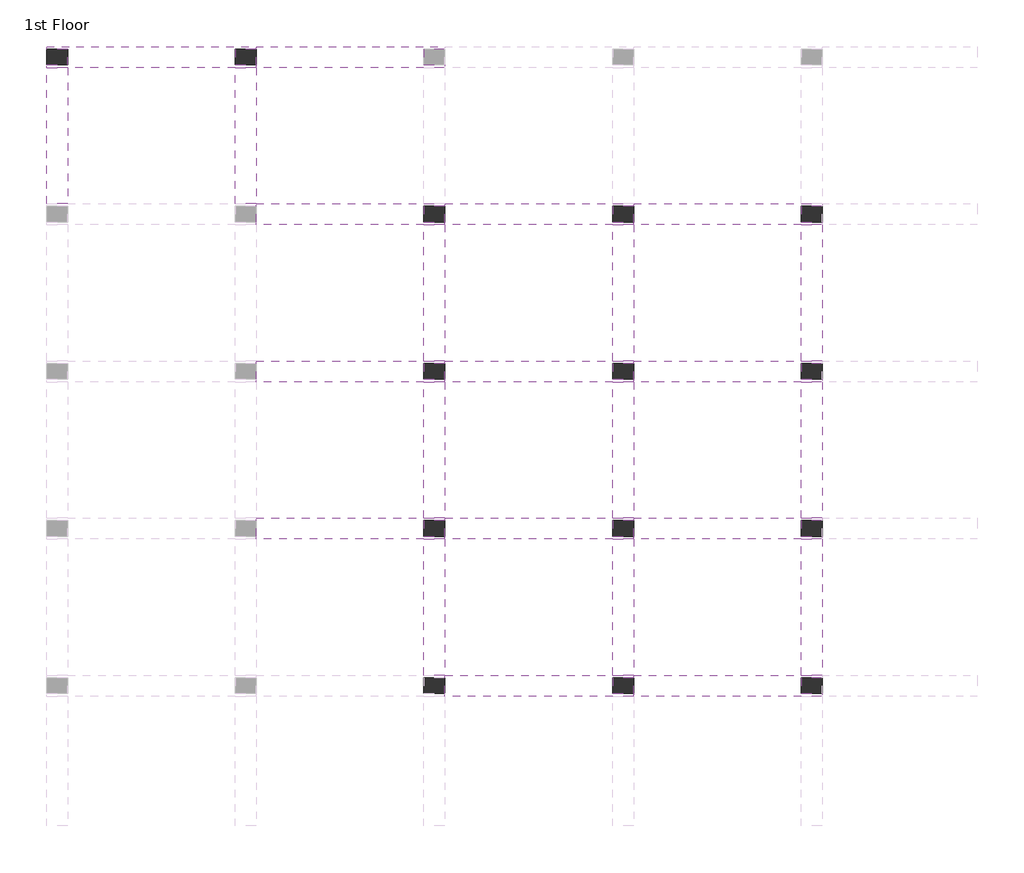
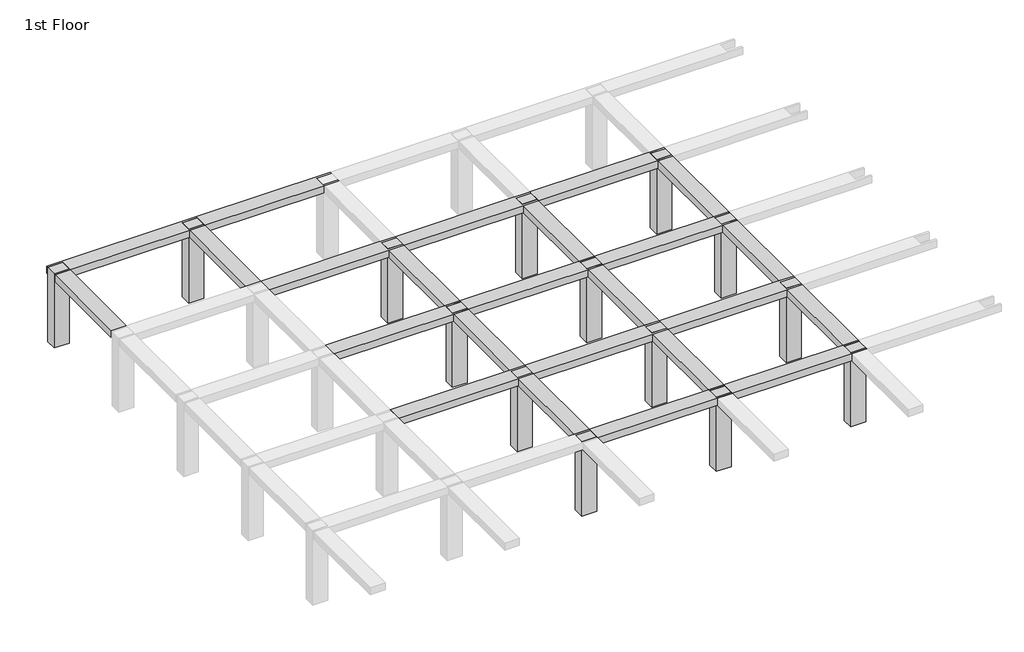
# One storey, part 2 of 3: 24 beams, 14 columns.
"""IFC4 building model written with IfcOpenShell, lengths in millimetres."""

from ifc_helpers import new_model, si_unit, frame, origin, place, context, project, spatial, polyline, outline, extrude, faceted_brep, element, save

model = new_model("IFC4")

# Units and contexts
model_context = context("Model", 3, world=origin())
ifc_project = project(units=[si_unit("LENGTHUNIT", "METRE", prefix="MILLI")], contexts=[model_context])

# Site, building, storey
site = spatial("IfcSite", under=ifc_project)
building = spatial("IfcBuilding", under=site)
storey = spatial("IfcBuildingStorey", under=building, Name="1st Floor", Elevation=3200.4)

# Beams
placement = place(None, origin())
element("IfcBeam", 1, ObjectType="Concrete-Rectangular Beam : 2' x2'", at=placement, inside=storey, context=model_context, shape_type="Brep", body=[
    faceted_brep([(-5646.474232, 1680.7831222, 6400.8), (-6256.074232, 1680.7831222, 6400.8), (-11132.874232, 1680.7831222, 6400.8), (-11132.874232, 1604.5831222, 6400.8), (-11132.874232, 1147.3831222, 6400.8), (-11132.874232, 1071.1831222, 6400.8), (-6256.074232, 1071.1831222, 6400.8), (-5646.474232, 1071.1831222, 6400.8), (-5646.474232, 1147.3831222, 6400.8), (-6256.074232, 1147.3831222, 6400.8), (-6256.074232, 1604.5831222, 6400.8), (-5646.474232, 1604.5831222, 6400.8), (-5646.474232, 1071.1831222, 6096.0), (-11132.874232, 1071.1831222, 6096.0), (-6256.074232, 1071.1831222, 6096.0), (-11132.874232, 1147.3831222, 6096.0), (-11132.874232, 1604.5831222, 6096.0), (-11132.874232, 1680.7831222, 6096.0), (-6256.074232, 1680.7831222, 6096.0), (-5646.474232, 1680.7831222, 6096.0), (-5646.474232, 1604.5831222, 6096.0), (-6256.074232, 1604.5831222, 6096.0), (-6256.074232, 1147.3831222, 6096.0), (-5646.474232, 1147.3831222, 6096.0)], [[[0, 1, 2, 3, 4, 5, 6, 7, 8, 9, 10, 11]], [[12, 7, 6, 5, 13, 14]], [[12, 14, 13, 15, 16, 17, 18, 19, 20, 21, 22, 23]], [[0, 19, 18, 17, 2, 1]], [[7, 12, 23, 8]], [[5, 4, 3, 2, 17, 16, 15, 13]], [[22, 9, 8, 23]], [[9, 22, 21, 10]], [[10, 21, 20, 11]], [[19, 0, 11, 20]]]),
])
element("IfcBeam", 2, ObjectType="Concrete-Rectangular Beam : 2' x2'", at=placement, inside=storey, context=model_context, shape_type="Brep", body=[
    faceted_brep([(-5646.474232, 1680.7831222, 6400.8), (-5646.474232, 1604.5831222, 6400.8), (-5646.474232, 1147.3831222, 6400.8), (-5646.474232, 1071.1831222, 6400.8), (-769.674232, 1071.1831222, 6400.8), (-160.074232, 1071.1831222, 6400.8), (-160.074232, 1147.3831222, 6400.8), (-769.674232, 1147.3831222, 6400.8), (-769.674232, 1604.5831222, 6400.8), (-160.074232, 1604.5831222, 6400.8), (-160.074232, 1680.7831222, 6400.8), (-769.674232, 1680.7831222, 6400.8), (-5646.474232, 1071.1831222, 6096.0), (-769.674232, 1071.1831222, 6096.0), (-160.074232, 1071.1831222, 6096.0), (-5646.474232, 1147.3831222, 6096.0), (-5646.474232, 1604.5831222, 6096.0), (-5646.474232, 1680.7831222, 6096.0), (-769.674232, 1680.7831222, 6096.0), (-160.074232, 1680.7831222, 6096.0), (-160.074232, 1604.5831222, 6096.0), (-769.674232, 1604.5831222, 6096.0), (-769.674232, 1147.3831222, 6096.0), (-160.074232, 1147.3831222, 6096.0)], [[[0, 1, 2, 3, 4, 5, 6, 7, 8, 9, 10, 11]], [[3, 12, 13, 14, 5, 4]], [[12, 15, 16, 17, 18, 19, 20, 21, 22, 23, 14, 13]], [[10, 19, 18, 17, 0, 11]], [[3, 2, 1, 0, 17, 16, 15, 12]], [[5, 14, 23, 6]], [[22, 7, 6, 23]], [[7, 22, 21, 8]], [[8, 21, 20, 9]], [[19, 10, 9, 20]]]),
])
element("IfcBeam", 3, ObjectType="Concrete-Rectangular Beam : 2' x2'", at=placement, inside=storey, context=model_context, shape_type="Brep", body=[
    faceted_brep([(-16619.274232, 6252.7831222, 6400.8), (-16619.274232, 6176.5831222, 6400.8), (-16619.274232, 5719.3831222, 6400.8), (-16619.274232, 5643.1831222, 6400.8), (-11742.474232, 5643.1831222, 6400.8), (-11132.874232, 5643.1831222, 6400.8), (-11132.874232, 5719.3831222, 6400.8), (-11742.474232, 5719.3831222, 6400.8), (-11742.474232, 6176.5831222, 6400.8), (-11132.874232, 6176.5831222, 6400.8), (-11132.874232, 6252.7831222, 6400.8), (-11742.474232, 6252.7831222, 6400.8), (-16619.274232, 5643.1831222, 6096.0), (-11742.474232, 5643.1831222, 6096.0), (-11132.874232, 5643.1831222, 6096.0), (-16619.274232, 5719.3831222, 6096.0), (-16619.274232, 6176.5831222, 6096.0), (-16619.274232, 6252.7831222, 6096.0), (-11742.474232, 6252.7831222, 6096.0), (-11132.874232, 6252.7831222, 6096.0), (-11132.874232, 6176.5831222, 6096.0), (-11742.474232, 6176.5831222, 6096.0), (-11742.474232, 5719.3831222, 6096.0), (-11132.874232, 5719.3831222, 6096.0)], [[[0, 1, 2, 3, 4, 5, 6, 7, 8, 9, 10, 11]], [[3, 12, 13, 14, 5, 4]], [[12, 15, 16, 17, 18, 19, 20, 21, 22, 23, 14, 13]], [[10, 19, 18, 17, 0, 11]], [[3, 2, 1, 0, 17, 16, 15, 12]], [[5, 14, 23, 6]], [[22, 7, 6, 23]], [[7, 22, 21, 8]], [[8, 21, 20, 9]], [[19, 10, 9, 20]]]),
])
element("IfcBeam", 4, ObjectType="Concrete-Rectangular Beam : 2' x2'", at=placement, inside=storey, context=model_context, shape_type="Brep", body=[
    faceted_brep([(-5646.474232, 6252.7831222, 6400.8), (-6256.074232, 6252.7831222, 6400.8), (-11132.874232, 6252.7831222, 6400.8), (-11132.874232, 6176.5831222, 6400.8), (-11132.874232, 5719.3831222, 6400.8), (-11132.874232, 5643.1831222, 6400.8), (-6256.074232, 5643.1831222, 6400.8), (-5646.474232, 5643.1831222, 6400.8), (-5646.474232, 5719.3831222, 6400.8), (-6256.074232, 5719.3831222, 6400.8), (-6256.074232, 6176.5831222, 6400.8), (-5646.474232, 6176.5831222, 6400.8), (-5646.474232, 5643.1831222, 6096.0), (-11132.874232, 5643.1831222, 6096.0), (-6256.074232, 5643.1831222, 6096.0), (-11132.874232, 5719.3831222, 6096.0), (-11132.874232, 6176.5831222, 6096.0), (-11132.874232, 6252.7831222, 6096.0), (-6256.074232, 6252.7831222, 6096.0), (-5646.474232, 6252.7831222, 6096.0), (-5646.474232, 6176.5831222, 6096.0), (-6256.074232, 6176.5831222, 6096.0), (-6256.074232, 5719.3831222, 6096.0), (-5646.474232, 5719.3831222, 6096.0)], [[[0, 1, 2, 3, 4, 5, 6, 7, 8, 9, 10, 11]], [[12, 7, 6, 5, 13, 14]], [[12, 14, 13, 15, 16, 17, 18, 19, 20, 21, 22, 23]], [[0, 19, 18, 17, 2, 1]], [[7, 12, 23, 8]], [[5, 4, 3, 2, 17, 16, 15, 13]], [[22, 9, 8, 23]], [[9, 22, 21, 10]], [[10, 21, 20, 11]], [[19, 0, 11, 20]]]),
])
element("IfcBeam", 5, ObjectType="Concrete-Rectangular Beam : 2' x2'", at=placement, inside=storey, context=model_context, shape_type="Brep", body=[
    faceted_brep([(-5646.474232, 6252.7831222, 6400.8), (-5646.474232, 6176.5831222, 6400.8), (-5646.474232, 5719.3831222, 6400.8), (-5646.474232, 5643.1831222, 6400.8), (-769.674232, 5643.1831222, 6400.8), (-160.074232, 5643.1831222, 6400.8), (-160.074232, 5719.3831222, 6400.8), (-769.674232, 5719.3831222, 6400.8), (-769.674232, 6176.5831222, 6400.8), (-160.074232, 6176.5831222, 6400.8), (-160.074232, 6252.7831222, 6400.8), (-769.674232, 6252.7831222, 6400.8), (-5646.474232, 5643.1831222, 6096.0), (-769.674232, 5643.1831222, 6096.0), (-160.074232, 5643.1831222, 6096.0), (-5646.474232, 5719.3831222, 6096.0), (-5646.474232, 6176.5831222, 6096.0), (-5646.474232, 6252.7831222, 6096.0), (-769.674232, 6252.7831222, 6096.0), (-160.074232, 6252.7831222, 6096.0), (-160.074232, 6176.5831222, 6096.0), (-769.674232, 6176.5831222, 6096.0), (-769.674232, 5719.3831222, 6096.0), (-160.074232, 5719.3831222, 6096.0)], [[[0, 1, 2, 3, 4, 5, 6, 7, 8, 9, 10, 11]], [[3, 12, 13, 14, 5, 4]], [[12, 15, 16, 17, 18, 19, 20, 21, 22, 23, 14, 13]], [[10, 19, 18, 17, 0, 11]], [[3, 2, 1, 0, 17, 16, 15, 12]], [[5, 14, 23, 6]], [[22, 7, 6, 23]], [[7, 22, 21, 8]], [[8, 21, 20, 9]], [[19, 10, 9, 20]]]),
])
element("IfcBeam", 6, ObjectType="Concrete-Rectangular Beam : 2' x2'", at=placement, inside=storey, context=model_context, shape_type="Brep", body=[
    faceted_brep([(-16619.274232, 10824.7831222, 6400.8), (-16619.274232, 10748.5831222, 6400.8), (-16619.274232, 10291.3831222, 6400.8), (-16619.274232, 10215.1831222, 6400.8), (-11742.474232, 10215.1831222, 6400.8), (-11132.874232, 10215.1831222, 6400.8), (-11132.874232, 10291.3831222, 6400.8), (-11742.474232, 10291.3831222, 6400.8), (-11742.474232, 10748.5831222, 6400.8), (-11132.874232, 10748.5831222, 6400.8), (-11132.874232, 10824.7831222, 6400.8), (-11742.474232, 10824.7831222, 6400.8), (-16619.274232, 10215.1831222, 6096.0), (-11742.474232, 10215.1831222, 6096.0), (-11132.874232, 10215.1831222, 6096.0), (-16619.274232, 10291.3831222, 6096.0), (-16619.274232, 10748.5831222, 6096.0), (-16619.274232, 10824.7831222, 6096.0), (-11742.474232, 10824.7831222, 6096.0), (-11132.874232, 10824.7831222, 6096.0), (-11132.874232, 10748.5831222, 6096.0), (-11742.474232, 10748.5831222, 6096.0), (-11742.474232, 10291.3831222, 6096.0), (-11132.874232, 10291.3831222, 6096.0)], [[[0, 1, 2, 3, 4, 5, 6, 7, 8, 9, 10, 11]], [[3, 12, 13, 14, 5, 4]], [[12, 15, 16, 17, 18, 19, 20, 21, 22, 23, 14, 13]], [[10, 19, 18, 17, 0, 11]], [[3, 2, 1, 0, 17, 16, 15, 12]], [[5, 14, 23, 6]], [[22, 7, 6, 23]], [[7, 22, 21, 8]], [[8, 21, 20, 9]], [[19, 10, 9, 20]]]),
])
element("IfcBeam", 7, ObjectType="Concrete-Rectangular Beam : 2' x2'", at=placement, inside=storey, context=model_context, shape_type="Brep", body=[
    faceted_brep([(-11132.874232, 10824.7831222, 6400.8), (-11132.874232, 10748.5831222, 6400.8), (-11132.874232, 10291.3831222, 6400.8), (-11132.874232, 10215.1831222, 6400.8), (-6256.074232, 10215.1831222, 6400.8), (-5646.474232, 10215.1831222, 6400.8), (-5646.474232, 10291.3831222, 6400.8), (-6256.074232, 10291.3831222, 6400.8), (-6256.074232, 10748.5831222, 6400.8), (-5646.474232, 10748.5831222, 6400.8), (-5646.474232, 10824.7831222, 6400.8), (-6256.074232, 10824.7831222, 6400.8), (-11132.874232, 10215.1831222, 6096.0), (-6256.074232, 10215.1831222, 6096.0), (-5646.474232, 10215.1831222, 6096.0), (-11132.874232, 10291.3831222, 6096.0), (-11132.874232, 10748.5831222, 6096.0), (-11132.874232, 10824.7831222, 6096.0), (-6256.074232, 10824.7831222, 6096.0), (-5646.474232, 10824.7831222, 6096.0), (-5646.474232, 10748.5831222, 6096.0), (-6256.074232, 10748.5831222, 6096.0), (-6256.074232, 10291.3831222, 6096.0), (-5646.474232, 10291.3831222, 6096.0)], [[[0, 1, 2, 3, 4, 5, 6, 7, 8, 9, 10, 11]], [[3, 12, 13, 14, 5, 4]], [[12, 15, 16, 17, 18, 19, 20, 21, 22, 23, 14, 13]], [[10, 19, 18, 17, 0, 11]], [[3, 2, 1, 0, 17, 16, 15, 12]], [[5, 14, 23, 6]], [[22, 7, 6, 23]], [[7, 22, 21, 8]], [[8, 21, 20, 9]], [[19, 10, 9, 20]]]),
])
element("IfcBeam", 8, ObjectType="Concrete-Rectangular Beam : 2' x2'", at=placement, inside=storey, context=model_context, shape_type="Brep", body=[
    faceted_brep([(-5646.474232, 10824.7831222, 6400.8), (-5646.474232, 10748.5831222, 6400.8), (-5646.474232, 10291.3831222, 6400.8), (-5646.474232, 10215.1831222, 6400.8), (-769.674232, 10215.1831222, 6400.8), (-160.074232, 10215.1831222, 6400.8), (-160.074232, 10291.3831222, 6400.8), (-769.674232, 10291.3831222, 6400.8), (-769.674232, 10748.5831222, 6400.8), (-160.074232, 10748.5831222, 6400.8), (-160.074232, 10824.7831222, 6400.8), (-769.674232, 10824.7831222, 6400.8), (-5646.474232, 10215.1831222, 6096.0), (-769.674232, 10215.1831222, 6096.0), (-160.074232, 10215.1831222, 6096.0), (-5646.474232, 10291.3831222, 6096.0), (-5646.474232, 10748.5831222, 6096.0), (-5646.474232, 10824.7831222, 6096.0), (-769.674232, 10824.7831222, 6096.0), (-160.074232, 10824.7831222, 6096.0), (-160.074232, 10748.5831222, 6096.0), (-769.674232, 10748.5831222, 6096.0), (-769.674232, 10291.3831222, 6096.0), (-160.074232, 10291.3831222, 6096.0)], [[[0, 1, 2, 3, 4, 5, 6, 7, 8, 9, 10, 11]], [[3, 12, 13, 14, 5, 4]], [[12, 15, 16, 17, 18, 19, 20, 21, 22, 23, 14, 13]], [[10, 19, 18, 17, 0, 11]], [[3, 2, 1, 0, 17, 16, 15, 12]], [[5, 14, 23, 6]], [[22, 7, 6, 23]], [[7, 22, 21, 8]], [[8, 21, 20, 9]], [[19, 10, 9, 20]]]),
])
element("IfcBeam", 9, ObjectType="Concrete-Rectangular Beam : 2' x2'", at=placement, inside=storey, context=model_context, shape_type="Brep", body=[
    faceted_brep([(-16619.274232, 15396.7831222, 6400.8), (-16619.274232, 15320.5831222, 6400.8), (-16619.274232, 14863.3831222, 6400.8), (-16619.274232, 14787.1831222, 6400.8), (-11742.474232, 14787.1831222, 6400.8), (-11132.874232, 14787.1831222, 6400.8), (-11132.874232, 14863.3831222, 6400.8), (-11742.474232, 14863.3831222, 6400.8), (-11742.474232, 15320.5831222, 6400.8), (-11132.874232, 15320.5831222, 6400.8), (-11132.874232, 15396.7831222, 6400.8), (-11742.474232, 15396.7831222, 6400.8), (-16619.274232, 14787.1831222, 6096.0), (-11742.474232, 14787.1831222, 6096.0), (-11132.874232, 14787.1831222, 6096.0), (-16619.274232, 14863.3831222, 6096.0), (-16619.274232, 15320.5831222, 6096.0), (-16619.274232, 15396.7831222, 6096.0), (-11742.474232, 15396.7831222, 6096.0), (-11132.874232, 15396.7831222, 6096.0), (-11132.874232, 15320.5831222, 6096.0), (-11742.474232, 15320.5831222, 6096.0), (-11742.474232, 14863.3831222, 6096.0), (-11132.874232, 14863.3831222, 6096.0)], [[[0, 1, 2, 3, 4, 5, 6, 7, 8, 9, 10, 11]], [[3, 12, 13, 14, 5, 4]], [[12, 15, 16, 17, 18, 19, 20, 21, 22, 23, 14, 13]], [[10, 19, 18, 17, 0, 11]], [[3, 2, 1, 0, 17, 16, 15, 12]], [[5, 14, 23, 6]], [[22, 7, 6, 23]], [[7, 22, 21, 8]], [[8, 21, 20, 9]], [[19, 10, 9, 20]]]),
])
element("IfcBeam", 10, ObjectType="Concrete-Rectangular Beam : 2' x2'", at=placement, inside=storey, context=model_context, shape_type="Brep", body=[
    faceted_brep([(-11132.874232, 15396.7831222, 6400.8), (-11132.874232, 15320.5831222, 6400.8), (-11132.874232, 14863.3831222, 6400.8), (-11132.874232, 14787.1831222, 6400.8), (-6256.074232, 14787.1831222, 6400.8), (-5646.474232, 14787.1831222, 6400.8), (-5646.474232, 14863.3831222, 6400.8), (-6256.074232, 14863.3831222, 6400.8), (-6256.074232, 15320.5831222, 6400.8), (-5646.474232, 15320.5831222, 6400.8), (-5646.474232, 15396.7831222, 6400.8), (-6256.074232, 15396.7831222, 6400.8), (-11132.874232, 14787.1831222, 6096.0), (-6256.074232, 14787.1831222, 6096.0), (-5646.474232, 14787.1831222, 6096.0), (-11132.874232, 14863.3831222, 6096.0), (-11132.874232, 15320.5831222, 6096.0), (-11132.874232, 15396.7831222, 6096.0), (-6256.074232, 15396.7831222, 6096.0), (-5646.474232, 15396.7831222, 6096.0), (-5646.474232, 15320.5831222, 6096.0), (-6256.074232, 15320.5831222, 6096.0), (-6256.074232, 14863.3831222, 6096.0), (-5646.474232, 14863.3831222, 6096.0)], [[[0, 1, 2, 3, 4, 5, 6, 7, 8, 9, 10, 11]], [[3, 12, 13, 14, 5, 4]], [[12, 15, 16, 17, 18, 19, 20, 21, 22, 23, 14, 13]], [[10, 19, 18, 17, 0, 11]], [[3, 2, 1, 0, 17, 16, 15, 12]], [[5, 14, 23, 6]], [[22, 7, 6, 23]], [[7, 22, 21, 8]], [[8, 21, 20, 9]], [[19, 10, 9, 20]]]),
])
element("IfcBeam", 11, ObjectType="Concrete-Rectangular Beam : 2' x2'", at=placement, inside=storey, context=model_context, shape_type="Brep", body=[
    faceted_brep([(-5646.474232, 15396.7831222, 6400.8), (-5646.474232, 15320.5831222, 6400.8), (-5646.474232, 14863.3831222, 6400.8), (-5646.474232, 14787.1831222, 6400.8), (-769.674232, 14787.1831222, 6400.8), (-160.074232, 14787.1831222, 6400.8), (-160.074232, 14863.3831222, 6400.8), (-769.674232, 14863.3831222, 6400.8), (-769.674232, 15320.5831222, 6400.8), (-160.074232, 15320.5831222, 6400.8), (-160.074232, 15396.7831222, 6400.8), (-769.674232, 15396.7831222, 6400.8), (-5646.474232, 14787.1831222, 6096.0), (-769.674232, 14787.1831222, 6096.0), (-160.074232, 14787.1831222, 6096.0), (-5646.474232, 14863.3831222, 6096.0), (-5646.474232, 15320.5831222, 6096.0), (-5646.474232, 15396.7831222, 6096.0), (-769.674232, 15396.7831222, 6096.0), (-160.074232, 15396.7831222, 6096.0), (-160.074232, 15320.5831222, 6096.0), (-769.674232, 15320.5831222, 6096.0), (-769.674232, 14863.3831222, 6096.0), (-160.074232, 14863.3831222, 6096.0)], [[[0, 1, 2, 3, 4, 5, 6, 7, 8, 9, 10, 11]], [[3, 12, 13, 14, 5, 4]], [[12, 15, 16, 17, 18, 19, 20, 21, 22, 23, 14, 13]], [[10, 19, 18, 17, 0, 11]], [[3, 2, 1, 0, 17, 16, 15, 12]], [[5, 14, 23, 6]], [[22, 7, 6, 23]], [[7, 22, 21, 8]], [[8, 21, 20, 9]], [[19, 10, 9, 20]]]),
])
element("IfcBeam", 12, ObjectType="Concrete-Rectangular Beam : 2' x2'", at=placement, inside=storey, context=model_context, shape_type="Brep", body=[
    faceted_brep([(-16619.274232, 19968.7831222, 6400.8), (-22715.274232, 19968.7831222, 6400.8), (-22715.274232, 19892.5831222, 6400.8), (-22105.674232, 19892.5831222, 6400.8), (-22105.674232, 19435.3831222, 6400.8), (-22715.274232, 19435.3831222, 6400.8), (-22715.274232, 19359.1831222, 6400.8), (-22105.674232, 19359.1831222, 6400.8), (-17228.874232, 19359.1831222, 6400.8), (-16619.274232, 19359.1831222, 6400.8), (-16619.274232, 19435.3831222, 6400.8), (-17228.874232, 19435.3831222, 6400.8), (-17228.874232, 19892.5831222, 6400.8), (-16619.274232, 19892.5831222, 6400.8), (-22715.274232, 19359.1831222, 6096.0), (-22105.674232, 19359.1831222, 6096.0), (-17228.874232, 19359.1831222, 6096.0), (-16619.274232, 19359.1831222, 6096.0), (-22715.274232, 19435.3831222, 6096.0), (-22105.674232, 19435.3831222, 6096.0), (-22105.674232, 19892.5831222, 6096.0), (-22715.274232, 19892.5831222, 6096.0), (-22715.274232, 19968.7831222, 6096.0), (-16619.274232, 19968.7831222, 6096.0), (-16619.274232, 19892.5831222, 6096.0), (-17228.874232, 19892.5831222, 6096.0), (-17228.874232, 19435.3831222, 6096.0), (-16619.274232, 19435.3831222, 6096.0)], [[[0, 1, 2, 3, 4, 5, 6, 7, 8, 9, 10, 11, 12, 13]], [[6, 14, 15, 16, 17, 9, 8, 7]], [[17, 16, 15, 14, 18, 19, 20, 21, 22, 23, 24, 25, 26, 27]], [[22, 1, 0, 23]], [[14, 6, 5, 18]], [[9, 17, 27, 10]], [[19, 4, 3, 20]], [[4, 19, 18, 5]], [[20, 3, 2, 21]], [[1, 22, 21, 2]], [[26, 11, 10, 27]], [[11, 26, 25, 12]], [[12, 25, 24, 13]], [[23, 0, 13, 24]]]),
])
element("IfcBeam", 13, ObjectType="Concrete-Rectangular Beam : 2' x2'", at=placement, inside=storey, context=model_context, shape_type="Brep", body=[
    faceted_brep([(-11132.874232, 19968.7831222, 6400.8), (-16619.274232, 19968.7831222, 6400.8), (-16619.274232, 19892.5831222, 6400.8), (-16619.274232, 19435.3831222, 6400.8), (-16619.274232, 19359.1831222, 6400.8), (-11742.474232, 19359.1831222, 6400.8), (-11132.874232, 19359.1831222, 6400.8), (-11132.874232, 19435.3831222, 6400.8), (-11742.474232, 19435.3831222, 6400.8), (-11742.474232, 19892.5831222, 6400.8), (-11132.874232, 19892.5831222, 6400.8), (-11132.874232, 19359.1831222, 6096.0), (-16619.274232, 19359.1831222, 6096.0), (-11742.474232, 19359.1831222, 6096.0), (-16619.274232, 19435.3831222, 6096.0), (-16619.274232, 19892.5831222, 6096.0), (-16619.274232, 19968.7831222, 6096.0), (-11132.874232, 19968.7831222, 6096.0), (-11132.874232, 19892.5831222, 6096.0), (-11742.474232, 19892.5831222, 6096.0), (-11742.474232, 19435.3831222, 6096.0), (-11132.874232, 19435.3831222, 6096.0)], [[[0, 1, 2, 3, 4, 5, 6, 7, 8, 9, 10]], [[11, 6, 5, 4, 12, 13]], [[11, 13, 12, 14, 15, 16, 17, 18, 19, 20, 21]], [[0, 17, 16, 1]], [[6, 11, 21, 7]], [[4, 3, 2, 1, 16, 15, 14, 12]], [[20, 8, 7, 21]], [[8, 20, 19, 9]], [[9, 19, 18, 10]], [[17, 0, 10, 18]]]),
])
element("IfcBeam", 14, ObjectType="Concrete-Rectangular Beam : 2' x2'", at=placement, inside=storey, context=model_context, shape_type="SweptSolid", body=[
    extrude(outline(polyline([(-22105.674232, 15396.7831222), (-22715.274232, 15396.7831222), (-22715.274232, 19359.1831222), (-22105.674232, 19359.1831222), (-22105.674232, 15396.7831222)])), frame((0.0, 0.0, 6096.0), z_axis=(0.0, 0.0, 1.0), x_axis=(1.0, 0.0, 0.0)), (0.0, 0.0, 1.0), 304.8),
])
element("IfcBeam", 15, ObjectType="Concrete-Rectangular Beam : 2' x2'", at=placement, inside=storey, context=model_context, shape_type="SweptSolid", body=[
    extrude(outline(polyline([(-16619.274232, 15396.7831222), (-17228.874232, 15396.7831222), (-17228.874232, 19359.1831222), (-16619.274232, 19359.1831222), (-16619.274232, 15396.7831222)])), frame((0.0, 0.0, 6096.0), z_axis=(0.0, 0.0, 1.0), x_axis=(1.0, 0.0, 0.0)), (0.0, 0.0, 1.0), 304.8),
])
element("IfcBeam", 16, ObjectType="Concrete-Rectangular Beam : 2' x2'", at=placement, inside=storey, context=model_context, shape_type="SweptSolid", body=[
    extrude(outline(polyline([(-11132.874232, 1680.7831222), (-11742.474232, 1680.7831222), (-11742.474232, 5643.1831222), (-11132.874232, 5643.1831222), (-11132.874232, 1680.7831222)])), frame((0.0, 0.0, 6096.0), z_axis=(0.0, 0.0, 1.0), x_axis=(1.0, 0.0, 0.0)), (0.0, 0.0, 1.0), 304.8),
])
element("IfcBeam", 17, ObjectType="Concrete-Rectangular Beam : 2' x2'", at=placement, inside=storey, context=model_context, shape_type="SweptSolid", body=[
    extrude(outline(polyline([(-11132.874232, 6252.7831222), (-11742.474232, 6252.7831222), (-11742.474232, 10215.1831222), (-11132.874232, 10215.1831222), (-11132.874232, 6252.7831222)])), frame((0.0, 0.0, 6096.0), z_axis=(0.0, 0.0, 1.0), x_axis=(1.0, 0.0, 0.0)), (0.0, 0.0, 1.0), 304.8),
])
element("IfcBeam", 18, ObjectType="Concrete-Rectangular Beam : 2' x2'", at=placement, inside=storey, context=model_context, shape_type="SweptSolid", body=[
    extrude(outline(polyline([(-11132.874232, 10824.7831222), (-11742.474232, 10824.7831222), (-11742.474232, 14787.1831222), (-11132.874232, 14787.1831222), (-11132.874232, 10824.7831222)])), frame((0.0, 0.0, 6096.0), z_axis=(0.0, 0.0, 1.0), x_axis=(1.0, 0.0, 0.0)), (0.0, 0.0, 1.0), 304.8),
])
element("IfcBeam", 19, ObjectType="Concrete-Rectangular Beam : 2' x2'", at=placement, inside=storey, context=model_context, shape_type="SweptSolid", body=[
    extrude(outline(polyline([(-5646.474232, 1680.7831222), (-6256.074232, 1680.7831222), (-6256.074232, 5643.1831222), (-5646.474232, 5643.1831222), (-5646.474232, 1680.7831222)])), frame((0.0, 0.0, 6096.0), z_axis=(0.0, 0.0, 1.0), x_axis=(1.0, 0.0, 0.0)), (0.0, 0.0, 1.0), 304.8),
])
element("IfcBeam", 20, ObjectType="Concrete-Rectangular Beam : 2' x2'", at=placement, inside=storey, context=model_context, shape_type="SweptSolid", body=[
    extrude(outline(polyline([(-5646.474232, 6252.7831222), (-6256.074232, 6252.7831222), (-6256.074232, 10215.1831222), (-5646.474232, 10215.1831222), (-5646.474232, 6252.7831222)])), frame((0.0, 0.0, 6096.0), z_axis=(0.0, 0.0, 1.0), x_axis=(1.0, 0.0, 0.0)), (0.0, 0.0, 1.0), 304.8),
])
element("IfcBeam", 21, ObjectType="Concrete-Rectangular Beam : 2' x2'", at=placement, inside=storey, context=model_context, shape_type="SweptSolid", body=[
    extrude(outline(polyline([(-5646.474232, 10824.7831222), (-6256.074232, 10824.7831222), (-6256.074232, 14787.1831222), (-5646.474232, 14787.1831222), (-5646.474232, 10824.7831222)])), frame((0.0, 0.0, 6096.0), z_axis=(0.0, 0.0, 1.0), x_axis=(1.0, 0.0, 0.0)), (0.0, 0.0, 1.0), 304.8),
])
element("IfcBeam", 22, ObjectType="Concrete-Rectangular Beam : 2' x2'", at=placement, inside=storey, context=model_context, shape_type="SweptSolid", body=[
    extrude(outline(polyline([(-769.674232, 5643.1831222), (-160.074232, 5643.1831222), (-160.074232, 1680.7831222), (-769.674232, 1680.7831222), (-769.674232, 5643.1831222)])), frame((0.0, 0.0, 6096.0), z_axis=(0.0, 0.0, 1.0), x_axis=(1.0, 0.0, 0.0)), (0.0, 0.0, 1.0), 304.8),
])
element("IfcBeam", 23, ObjectType="Concrete-Rectangular Beam : 2' x2'", at=placement, inside=storey, context=model_context, shape_type="SweptSolid", body=[
    extrude(outline(polyline([(-160.074232, 6252.7831222), (-769.674232, 6252.7831222), (-769.674232, 10215.1831222), (-160.074232, 10215.1831222), (-160.074232, 6252.7831222)])), frame((0.0, 0.0, 6096.0), z_axis=(0.0, 0.0, 1.0), x_axis=(1.0, 0.0, 0.0)), (0.0, 0.0, 1.0), 304.8),
])
element("IfcBeam", 24, ObjectType="Concrete-Rectangular Beam : 2' x2'", at=placement, inside=storey, context=model_context, shape_type="SweptSolid", body=[
    extrude(outline(polyline([(-769.674232, 14787.1831222), (-160.074232, 14787.1831222), (-160.074232, 10824.7831222), (-769.674232, 10824.7831222), (-769.674232, 14787.1831222)])), frame((0.0, 0.0, 6096.0), z_axis=(0.0, 0.0, 1.0), x_axis=(1.0, 0.0, 0.0)), (0.0, 0.0, 1.0), 304.8),
])

# Columns
element("IfcColumn", 25, ObjectType="Concrete-Rectangular-Column : 12 x 18", at=placement, inside=storey, context=model_context, shape_type="SweptSolid", body=[
    extrude(outline(polyline([(-11132.874232, 1604.5831222), (-11132.874232, 1147.3831222), (-11742.474232, 1147.3831222), (-11742.474232, 1604.5831222), (-11132.874232, 1604.5831222)])), frame((0.0, 0.0, 3200.4), z_axis=(0.0, 0.0, 1.0), x_axis=(1.0, 0.0, 0.0)), (0.0, 0.0, 1.0), 3200.4),
])
element("IfcColumn", 26, ObjectType="Concrete-Rectangular-Column : 12 x 18", at=placement, inside=storey, context=model_context, shape_type="SweptSolid", body=[
    extrude(outline(polyline([(-5646.474232, 1604.5831222), (-5646.474232, 1147.3831222), (-6256.074232, 1147.3831222), (-6256.074232, 1604.5831222), (-5646.474232, 1604.5831222)])), frame((0.0, 0.0, 3200.4), z_axis=(0.0, 0.0, 1.0), x_axis=(1.0, 0.0, 0.0)), (0.0, 0.0, 1.0), 3200.4),
])
element("IfcColumn", 27, ObjectType="Concrete-Rectangular-Column : 12 x 18", at=placement, inside=storey, context=model_context, shape_type="SweptSolid", body=[
    extrude(outline(polyline([(-160.074232, 1604.5831222), (-160.074232, 1147.3831222), (-769.674232, 1147.3831222), (-769.674232, 1604.5831222), (-160.074232, 1604.5831222)])), frame((0.0, 0.0, 3200.4), z_axis=(0.0, 0.0, 1.0), x_axis=(1.0, 0.0, 0.0)), (0.0, 0.0, 1.0), 3200.4),
])
element("IfcColumn", 28, ObjectType="Concrete-Rectangular-Column : 12 x 18", at=placement, inside=storey, context=model_context, shape_type="SweptSolid", body=[
    extrude(outline(polyline([(-11132.874232, 6176.5831222), (-11132.874232, 5719.3831222), (-11742.474232, 5719.3831222), (-11742.474232, 6176.5831222), (-11132.874232, 6176.5831222)])), frame((0.0, 0.0, 3200.4), z_axis=(0.0, 0.0, 1.0), x_axis=(1.0, 0.0, 0.0)), (0.0, 0.0, 1.0), 3200.4),
])
element("IfcColumn", 29, ObjectType="Concrete-Rectangular-Column : 12 x 18", at=placement, inside=storey, context=model_context, shape_type="SweptSolid", body=[
    extrude(outline(polyline([(-5646.474232, 6176.5831222), (-5646.474232, 5719.3831222), (-6256.074232, 5719.3831222), (-6256.074232, 6176.5831222), (-5646.474232, 6176.5831222)])), frame((0.0, 0.0, 3200.4), z_axis=(0.0, 0.0, 1.0), x_axis=(1.0, 0.0, 0.0)), (0.0, 0.0, 1.0), 3200.4),
])
element("IfcColumn", 30, ObjectType="Concrete-Rectangular-Column : 12 x 18", at=placement, inside=storey, context=model_context, shape_type="SweptSolid", body=[
    extrude(outline(polyline([(-160.074232, 6176.5831222), (-160.074232, 5719.3831222), (-769.674232, 5719.3831222), (-769.674232, 6176.5831222), (-160.074232, 6176.5831222)])), frame((0.0, 0.0, 3200.4), z_axis=(0.0, 0.0, 1.0), x_axis=(1.0, 0.0, 0.0)), (0.0, 0.0, 1.0), 3200.4),
])
element("IfcColumn", 31, ObjectType="Concrete-Rectangular-Column : 12 x 18", at=placement, inside=storey, context=model_context, shape_type="SweptSolid", body=[
    extrude(outline(polyline([(-11132.874232, 10748.5831222), (-11132.874232, 10291.3831222), (-11742.474232, 10291.3831222), (-11742.474232, 10748.5831222), (-11132.874232, 10748.5831222)])), frame((0.0, 0.0, 3200.4), z_axis=(0.0, 0.0, 1.0), x_axis=(1.0, 0.0, 0.0)), (0.0, 0.0, 1.0), 3200.4),
])
element("IfcColumn", 32, ObjectType="Concrete-Rectangular-Column : 12 x 18", at=placement, inside=storey, context=model_context, shape_type="SweptSolid", body=[
    extrude(outline(polyline([(-5646.474232, 10748.5831222), (-5646.474232, 10291.3831222), (-6256.074232, 10291.3831222), (-6256.074232, 10748.5831222), (-5646.474232, 10748.5831222)])), frame((0.0, 0.0, 3200.4), z_axis=(0.0, 0.0, 1.0), x_axis=(1.0, 0.0, 0.0)), (0.0, 0.0, 1.0), 3200.4),
])
element("IfcColumn", 33, ObjectType="Concrete-Rectangular-Column : 12 x 18", at=placement, inside=storey, context=model_context, shape_type="SweptSolid", body=[
    extrude(outline(polyline([(-160.074232, 10748.5831222), (-160.074232, 10291.3831222), (-769.674232, 10291.3831222), (-769.674232, 10748.5831222), (-160.074232, 10748.5831222)])), frame((0.0, 0.0, 3200.4), z_axis=(0.0, 0.0, 1.0), x_axis=(1.0, 0.0, 0.0)), (0.0, 0.0, 1.0), 3200.4),
])
element("IfcColumn", 34, ObjectType="Concrete-Rectangular-Column : 12 x 18", at=placement, inside=storey, context=model_context, shape_type="SweptSolid", body=[
    extrude(outline(polyline([(-11132.874232, 15320.5831222), (-11132.874232, 14863.3831222), (-11742.474232, 14863.3831222), (-11742.474232, 15320.5831222), (-11132.874232, 15320.5831222)])), frame((0.0, 0.0, 3200.4), z_axis=(0.0, 0.0, 1.0), x_axis=(1.0, 0.0, 0.0)), (0.0, 0.0, 1.0), 3200.4),
])
element("IfcColumn", 35, ObjectType="Concrete-Rectangular-Column : 12 x 18", at=placement, inside=storey, context=model_context, shape_type="SweptSolid", body=[
    extrude(outline(polyline([(-5646.474232, 15320.5831222), (-5646.474232, 14863.3831222), (-6256.074232, 14863.3831222), (-6256.074232, 15320.5831222), (-5646.474232, 15320.5831222)])), frame((0.0, 0.0, 3200.4), z_axis=(0.0, 0.0, 1.0), x_axis=(1.0, 0.0, 0.0)), (0.0, 0.0, 1.0), 3200.4),
])
element("IfcColumn", 36, ObjectType="Concrete-Rectangular-Column : 12 x 18", at=placement, inside=storey, context=model_context, shape_type="SweptSolid", body=[
    extrude(outline(polyline([(-160.074232, 15320.5831222), (-160.074232, 14863.3831222), (-769.674232, 14863.3831222), (-769.674232, 15320.5831222), (-160.074232, 15320.5831222)])), frame((0.0, 0.0, 3200.4), z_axis=(0.0, 0.0, 1.0), x_axis=(1.0, 0.0, 0.0)), (0.0, 0.0, 1.0), 3200.4),
])
element("IfcColumn", 37, ObjectType="Concrete-Rectangular-Column : 12 x 18", at=placement, inside=storey, context=model_context, shape_type="SweptSolid", body=[
    extrude(outline(polyline([(-22105.674232, 19892.5831222), (-22105.674232, 19435.3831222), (-22715.274232, 19435.3831222), (-22715.274232, 19892.5831222), (-22105.674232, 19892.5831222)])), frame((0.0, 0.0, 3200.4), z_axis=(0.0, 0.0, 1.0), x_axis=(1.0, 0.0, 0.0)), (0.0, 0.0, 1.0), 3200.4),
])
element("IfcColumn", 38, ObjectType="Concrete-Rectangular-Column : 12 x 18", at=placement, inside=storey, context=model_context, shape_type="SweptSolid", body=[
    extrude(outline(polyline([(-16619.274232, 19892.5831222), (-16619.274232, 19435.3831222), (-17228.874232, 19435.3831222), (-17228.874232, 19892.5831222), (-16619.274232, 19892.5831222)])), frame((0.0, 0.0, 3200.4), z_axis=(0.0, 0.0, 1.0), x_axis=(1.0, 0.0, 0.0)), (0.0, 0.0, 1.0), 3200.4),
])

save(model, "model.ifc")

# Revit data of these elements
# Type "Concrete-Rectangular Beam : 2' x2'"
#   Assembly Code = "B10"
#   Length [instance default] = 5' - 0"
#   b = 2' - 0"
#   h = 1' - 0"
#   Structural Material [instance default] = Concrete, Cast-in-Place gray
# Type "Concrete-Rectangular-Column : 12 x 18"
#   Assembly Code = "B10"
#   b = 2' - 0"
#   h = 1' - 6"
#   Structural Material [instance default] = Concrete, Cast-in-Place gray
# Elements 1, 2, 3, 4, 5, 6, 7, 8, 9, 10, 11, 12, 13, 14, 15, 16, 17, 18, 19, 20, 21, 22, 23, 24 (IfcBeam, "Concrete-Rectangular Beam : 2' x2'")
#   Structural Material = Concrete, Precast (2)
#   Phase Created = New Construction
#   Materials on its faces: "Concrete, Precast (2)"
# Elements 25, 26, 27, 28, 29, 30, 31, 32, 33, 34, 35, 36, 37, 38 (IfcColumn, "Concrete-Rectangular-Column : 12 x 18")
#   Phase Created = New Construction
#   Materials on its faces: "Concrete, Cast-in-Place gray"
# Materials
#   "Concrete, Cast-in-Place gray": class "Concrete", colour RGB 192 192 192, transparency 0, Description = "Cast-in-place concrete", Cost = 0
#   "Concrete, Precast (2)": class "Concrete", colour RGB 198 187 187, transparency 0, Description = "Precast concrete", Cost = 0
